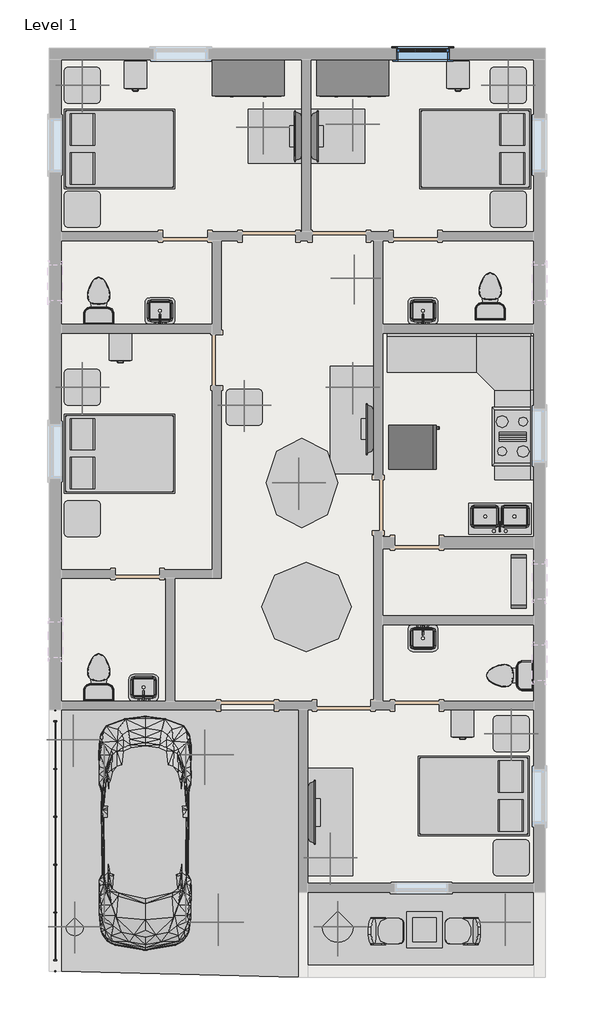
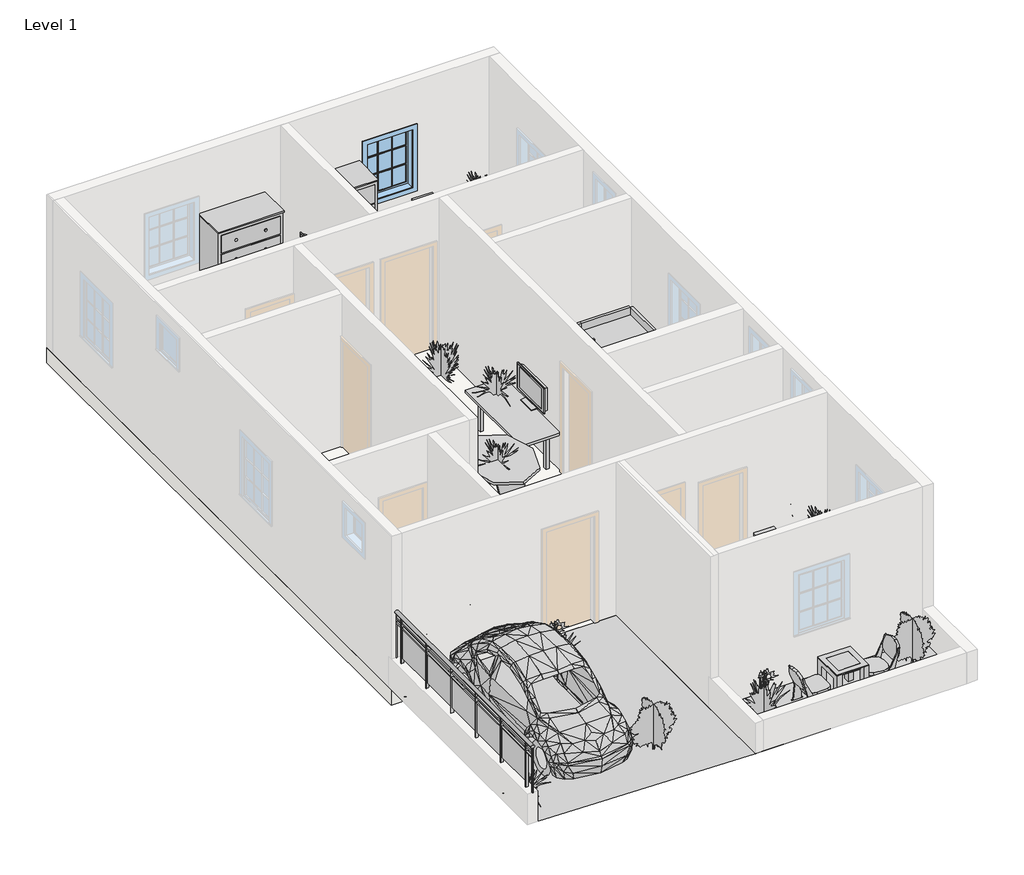
# One storey, part 2 of 2: 34 furniture elements, 17 geographic elements, 13 flow terminals, 5 proxies, 1 railing, 1 slab, 1 window.
"""IFC4 building model written with IfcOpenShell, lengths in millimetres."""

from ifc_helpers import new_model, si_unit, point, frame, origin, place, context, project, spatial, polyline, ellipse_curve, trimmed, outline, extrude, triangles, transform, mapped, element, save
from ifc_brep_helpers import plane_surface, extruded_surface, advanced_brep
from components import proxy_bb1e6e30, rpc_beetle_rpc_beetle_3ce7ba48, proxy_a13a33b2, flow_terminal_accce45a, flow_terminal_a53be723, flow_terminal_62a433f7, toilet_domestic_3d_toilet_domestic_3d_f7549cf7, toilet_domestic_3d_toilet_domestic_3d_183bbd19, furniture_c8abb964, furniture_bb55ed6b, furniture_9fa109b2, furniture_3d1d9cbc, furniture_417d203a, furniture_56245f3a, furniture_7a3aaa4f, furniture_b5c51a22, furniture_bbcc68ce, furniture_743965d2, furniture_31d08a24, furniture_4d44e21c, furniture_a5b052b6, furniture_125de5a1, rpc_plant_tropical_55f6ff97, rpc_plant_tropical_agave_1_5_93a2a214, rpc_plant_tropical_dagger_2_80c14bd7, rpc_plant_tropical_jungle_flame_3_9c4808c2, window_29c06734

model = new_model("IFC4")

# Units and contexts
model_context = context("Model", 3, world=origin())
ifc_project = project(units=[si_unit("LENGTHUNIT", "METRE", prefix="MILLI")], contexts=[model_context])

# Site, building, storey
site = spatial("IfcSite", under=ifc_project)
building = spatial("IfcBuilding", under=site)
storey = spatial("IfcBuildingStorey", under=building, Name="Level 1", Elevation=0.0)

# Proxies
placement = place(None, origin())
element("IfcBuildingElementProxy", 1, Name="Building Element Proxy", at=placement, inside=storey, context=model_context, shape_type="Tessellation", body=[
    triangles([(-16415.7270721, 2158.1188522, 0.0), (-12173.9266846, 2158.1188522, 0.0), (-12173.9266846, -2388.4812447, 0.0), (-16212.5266846, -2286.8811962, 0.0)], [[1, 4, 2], [3, 2, 4]], closed=False),
])
element("IfcBuildingElementProxy", 2, Name="Building Element Proxy", at=placement, inside=storey, context=model_context, shape_type="Tessellation", body=[
    triangles([(-12173.9266846, -940.6812447, 0.0), (-7982.9266846, -940.6812447, 0.0), (-7982.9266846, -2388.4812447, 0.0), (-12173.9266846, -2388.4812447, 0.0)], [[1, 4, 2], [3, 2, 4]], closed=False),
])
proxy_shape = proxy_bb1e6e30(model_context)
element("IfcBuildingElementProxy", 3, Name="Cook Top-4 Unit : 36\" x 20\"", ObjectType="Cook Top-4 Unit : 36\" x 20\"", at=placement, inside=storey, context=model_context, shape_type="MappedRepresentation", body=[
    mapped(proxy_shape, transform((-8541.7267032, 6806.3187882, 0.0), x_axis=(0.0, -1.0000000000000004, 0.0), y_axis=(1.0000000000000004, 0.0, 0.0), z_axis=(0.0, 0.0, 1.0))),
])
rpc_beetle_rpc_beetle_shape = rpc_beetle_rpc_beetle_3ce7ba48(model_context)
element("IfcBuildingElementProxy", 4, Name="RPC Beetle : RPC Beetle", ObjectType="RPC Beetle : RPC Beetle", at=placement, inside=storey, context=model_context, shape_type="MappedRepresentation", body=[
    mapped(rpc_beetle_rpc_beetle_shape, transform((-14790.1267032, 1294.5187882, 0.0), x_axis=(-1.0, 0.0, 0.0), y_axis=(0.0, -1.0, 0.0), z_axis=(0.0, 0.0, 1.0))),
])
proxy_2_shape = proxy_a13a33b2(model_context)
element("IfcBuildingElementProxy", 5, Name="Refrigerator : 30\" x 32\" RH", ObjectType="Refrigerator : 30\" x 32\" RH", at=placement, inside=storey, context=model_context, shape_type="MappedRepresentation", body=[
    mapped(proxy_2_shape, transform((-10260.9892032, 6620.9698167, 0.0), x_axis=(0.0, 1.0000000000000002, 0.0), y_axis=(-1.0000000000000002, 0.0, 0.0), z_axis=(0.0, 0.0, 1.0))),
])

# Flow terminals
flow_terminal_shape = flow_terminal_accce45a(model_context)
element("IfcFlowTerminal", 6, ObjectType="Floor Drain - Round : 5\" Strainer - 2\" Drain", at=placement, inside=storey, context=model_context, shape_type="MappedRepresentation", body=[
    mapped(flow_terminal_shape, transform((-15933.1267032, 9854.3187882, 0.0), x_axis=(1.0, 0.0, 0.0), y_axis=(0.0, 1.0, 0.0), z_axis=(0.0, 0.0, 1.0))),
])
element("IfcFlowTerminal", 7, ObjectType="Floor Drain - Round : 5\" Strainer - 2\" Drain", at=placement, inside=storey, context=model_context, shape_type="MappedRepresentation", body=[
    mapped(flow_terminal_shape, transform((-9329.1267032, 9828.9187882, 0.0), x_axis=(1.0, 0.0, 0.0), y_axis=(0.0, 1.0, 0.0), z_axis=(0.0, 0.0, 1.0))),
])
element("IfcFlowTerminal", 8, ObjectType="Floor Drain - Round : 5\" Strainer - 2\" Drain", at=placement, inside=storey, context=model_context, shape_type="MappedRepresentation", body=[
    mapped(flow_terminal_shape, transform((-15704.5267032, 3910.7187882, 0.0), x_axis=(1.0, 0.0, 0.0), y_axis=(0.0, 1.0, 0.0), z_axis=(0.0, 0.0, 1.0))),
])
element("IfcFlowTerminal", 9, ObjectType="Floor Drain - Round : 5\" Strainer - 2\" Drain", at=placement, inside=storey, context=model_context, shape_type="MappedRepresentation", body=[
    mapped(flow_terminal_shape, transform((-9252.9267032, 3351.9187882, 0.0), x_axis=(1.0, 0.0, 0.0), y_axis=(0.0, 1.0, 0.0), z_axis=(0.0, 0.0, 1.0))),
])
flow_terminal_2_shape = flow_terminal_a53be723(model_context)
element("IfcFlowTerminal", 10, ObjectType="Sink Kitchen-Double : 42\" x 21\"", at=placement, inside=storey, context=model_context, shape_type="MappedRepresentation", body=[
    mapped(flow_terminal_2_shape, transform((-8741.9374626, 5411.6641893, 0.0), x_axis=(-1.0000000000000004, 0.0, 0.0), y_axis=(0.0, -1.0000000000000004, 0.0), z_axis=(0.0, 0.0, 1.0))),
])
flow_terminal_3_shape = flow_terminal_62a433f7(model_context)
element("IfcFlowTerminal", 11, ObjectType="Sink Vanity-Square : 20\" x 18\"", at=placement, inside=storey, context=model_context, shape_type="MappedRepresentation", body=[
    mapped(flow_terminal_3_shape, transform((-14520.4374626, 8891.4641893, 0.0), x_axis=(-0.9999999999999999, 0.0, 0.0), y_axis=(0.0, -0.9999999999999999, 0.0), z_axis=(0.0, 0.0, 1.0))),
])
element("IfcFlowTerminal", 12, ObjectType="Sink Vanity-Square : 20\" x 18\"", at=placement, inside=storey, context=model_context, shape_type="MappedRepresentation", body=[
    mapped(flow_terminal_3_shape, transform((-10050.0374626, 8891.4641893, 0.0), x_axis=(-1.0, 0.0, 0.0), y_axis=(0.0, -1.0, 0.0), z_axis=(0.0, 0.0, 1.0))),
])
element("IfcFlowTerminal", 13, ObjectType="Sink Vanity-Square : 20\" x 18\"", at=placement, inside=storey, context=model_context, shape_type="MappedRepresentation", body=[
    mapped(flow_terminal_3_shape, transform((-14799.8374626, 2490.6641893, 0.0), x_axis=(-1.0000000000000002, 0.0, 0.0), y_axis=(0.0, -1.0000000000000002, 0.0), z_axis=(0.0, 0.0, 1.0))),
])
element("IfcFlowTerminal", 14, ObjectType="Sink Vanity-Square : 20\" x 18\"", at=placement, inside=storey, context=model_context, shape_type="MappedRepresentation", body=[
    mapped(flow_terminal_3_shape, transform((-10081.4159437, 3425.7733871, 0.0), x_axis=(1.0, 0.0, 0.0), y_axis=(0.0, 1.0, 0.0), z_axis=(0.0, 0.0, 1.0))),
])
toilet_domestic_3d_toilet_domestic_3d_shape = toilet_domestic_3d_toilet_domestic_3d_f7549cf7(model_context)
toilet_domestic_3d_toilet_domestic_3d_2_shape = toilet_domestic_3d_toilet_domestic_3d_183bbd19(model_context)
element("IfcFlowTerminal", 15, ObjectType="Toilet-Domestic-3D : Toilet-Domestic-3D", at=placement, inside=storey, context=model_context, shape_type="MappedRepresentation", body=[
    mapped(toilet_domestic_3d_toilet_domestic_3d_shape, transform((-15577.5267032, 9206.0148155, 0.0), x_axis=(-1.0000000000000002, 0.0, 0.0), y_axis=(0.0, -1.0000000000000002, 0.0), z_axis=(0.0, 0.0, 1.0))),
    mapped(toilet_domestic_3d_toilet_domestic_3d_2_shape, transform((-15577.5267032, 9206.0148155, 0.0), x_axis=(-1.0000000000000002, 0.0, 0.0), y_axis=(0.0, -1.0000000000000002, 0.0), z_axis=(0.0, 0.0, 1.0))),
])
element("IfcFlowTerminal", 16, ObjectType="Toilet-Domestic-3D : Toilet-Domestic-3D", at=placement, inside=storey, context=model_context, shape_type="MappedRepresentation", body=[
    mapped(toilet_domestic_3d_toilet_domestic_3d_shape, transform((-8922.7267032, 9282.2148155, 0.0), x_axis=(-0.9999999999999998, 0.0, 0.0), y_axis=(0.0, -0.9999999999999998, 0.0), z_axis=(0.0, 0.0, 1.0))),
    mapped(toilet_domestic_3d_toilet_domestic_3d_2_shape, transform((-8922.7267032, 9282.2148155, 0.0), x_axis=(-0.9999999999999998, 0.0, 0.0), y_axis=(0.0, -0.9999999999999998, 0.0), z_axis=(0.0, 0.0, 1.0))),
])
element("IfcFlowTerminal", 17, ObjectType="Toilet-Domestic-3D : Toilet-Domestic-3D", at=placement, inside=storey, context=model_context, shape_type="MappedRepresentation", body=[
    mapped(toilet_domestic_3d_toilet_domestic_3d_shape, transform((-15577.5267032, 2805.2148155, 0.0), x_axis=(-1.0000000000000002, 0.0, 0.0), y_axis=(0.0, -1.0000000000000002, 0.0), z_axis=(0.0, 0.0, 1.0))),
    mapped(toilet_domestic_3d_toilet_domestic_3d_2_shape, transform((-15577.5267032, 2805.2148155, 0.0), x_axis=(-1.0000000000000002, 0.0, 0.0), y_axis=(0.0, -1.0000000000000002, 0.0), z_axis=(0.0, 0.0, 1.0))),
])
element("IfcFlowTerminal", 18, ObjectType="Toilet-Domestic-3D : Toilet-Domestic-3D", at=placement, inside=storey, context=model_context, shape_type="MappedRepresentation", body=[
    mapped(toilet_domestic_3d_toilet_domestic_3d_shape, transform((-8680.8227305, 2742.3187882, 0.0), x_axis=(0.0, -1.0000000000000002, 0.0), y_axis=(1.0000000000000002, 0.0, 0.0), z_axis=(0.0, 0.0, 1.0))),
    mapped(toilet_domestic_3d_toilet_domestic_3d_2_shape, transform((-8680.8227305, 2742.3187882, 0.0), x_axis=(0.0, -1.0000000000000002, 0.0), y_axis=(1.0000000000000002, 0.0, 0.0), z_axis=(0.0, 0.0, 1.0))),
])

# Furniture
furniture_shape = furniture_c8abb964(model_context)
element("IfcFurniture", 19, ObjectType="Bed-Box : Double 53\" x 74\"", at=placement, inside=storey, context=model_context, shape_type="MappedRepresentation", body=[
    mapped(furniture_shape, transform((-15456.3562114, 11356.6663292, 0.0), x_axis=(0.0, 1.0, 0.0), y_axis=(-1.0, 0.0, 0.0), z_axis=(0.0, 0.0, 1.0))),
])
element("IfcFurniture", 20, ObjectType="Bed-Box : Double 53\" x 74\"", at=placement, inside=storey, context=model_context, shape_type="MappedRepresentation", body=[
    mapped(furniture_shape, transform((-8942.297195, 12034.9712472, 0.0), x_axis=(0.0, -1.0, 0.0), y_axis=(1.0, 0.0, 0.0), z_axis=(0.0, 0.0, 1.0))),
])
element("IfcFurniture", 21, ObjectType="Bed-Box : Double 53\" x 74\"", at=placement, inside=storey, context=model_context, shape_type="MappedRepresentation", body=[
    mapped(furniture_shape, transform((-15456.3562114, 6175.0663292, 0.0), x_axis=(0.0, 1.0, 0.0), y_axis=(-1.0, 0.0, 0.0), z_axis=(0.0, 0.0, 1.0))),
])
element("IfcFurniture", 22, ObjectType="Bed-Box : Double 53\" x 74\"", at=placement, inside=storey, context=model_context, shape_type="MappedRepresentation", body=[
    mapped(furniture_shape, transform((-8967.697195, 1036.7712472, 0.0), x_axis=(0.0, -1.0, 0.0), y_axis=(1.0, 0.0, 0.0), z_axis=(0.0, 0.0, 1.0))),
])
furniture_2_shape = furniture_bb55ed6b(model_context)
element("IfcFurniture", 23, ObjectType="Cabinet-File 2 Drawer : 15\" x 18\"", at=placement, inside=storey, context=model_context, shape_type="MappedRepresentation", body=[
    mapped(furniture_2_shape, transform((-14827.3302561, 13095.2530883, 0.0), x_axis=(1.0, 0.0, 0.0), y_axis=(0.0, 1.0, 0.0), z_axis=(0.0, 0.0, 1.0))),
])
element("IfcFurniture", 24, ObjectType="Cabinet-File 2 Drawer : 15\" x 18\"", at=placement, inside=storey, context=model_context, shape_type="MappedRepresentation", body=[
    mapped(furniture_2_shape, transform((-9340.9302561, 13095.2530883, 0.0), x_axis=(1.0, 0.0, 0.0), y_axis=(0.0, 1.0, 0.0), z_axis=(0.0, 0.0, 1.0))),
])
element("IfcFurniture", 25, ObjectType="Cabinet-File 2 Drawer : 15\" x 18\"", at=placement, inside=storey, context=model_context, shape_type="MappedRepresentation", body=[
    mapped(furniture_2_shape, transform((-9264.7302561, 2071.6530883, 0.0), x_axis=(1.0, 0.0, 0.0), y_axis=(0.0, 1.0, 0.0), z_axis=(0.0, 0.0, 1.0))),
])
element("IfcFurniture", 26, ObjectType="Cabinet-File 2 Drawer : 15\" x 18\"", at=placement, inside=storey, context=model_context, shape_type="MappedRepresentation", body=[
    mapped(furniture_2_shape, transform((-15081.3302561, 8472.4530883, 0.0), x_axis=(1.0, 0.0, 0.0), y_axis=(0.0, 1.0, 0.0), z_axis=(0.0, 0.0, 1.0))),
])
furniture_3_shape = furniture_9fa109b2(model_context)
element("IfcFurniture", 27, ObjectType="Dresser : 48\" x 72\" x 24\"", at=placement, inside=storey, context=model_context, shape_type="MappedRepresentation", body=[
    mapped(furniture_3_shape, transform((-12768.3334433, 13265.4817423, 0.0), x_axis=(1.0, 0.0, 0.0), y_axis=(0.0, 1.0, 0.0), z_axis=(0.0, 0.0, 1.0))),
])
element("IfcFurniture", 28, ObjectType="Dresser : 48\" x 72\" x 24\"", at=placement, inside=storey, context=model_context, shape_type="MappedRepresentation", body=[
    mapped(furniture_3_shape, transform((-10990.3334433, 13265.4817423, 0.0), x_axis=(1.0, 0.0, 0.0), y_axis=(0.0, 1.0, 0.0), z_axis=(0.0, 0.0, 1.0))),
])
furniture_4_shape = furniture_3d1d9cbc(model_context)
element("IfcFurniture", 29, ObjectType="Seating-Auditorium : 18\" x 24\" x 30\"", at=placement, inside=storey, context=model_context, shape_type="MappedRepresentation", body=[
    mapped(furniture_4_shape, transform((-9190.0512933, -1761.8090807, 0.0), x_axis=(0.0, 1.0000000000000002, 0.0), y_axis=(-1.0000000000000002, 0.0, 0.0), z_axis=(0.0, 0.0, 1.0))),
])
element("IfcFurniture", 30, ObjectType="Seating-Auditorium : 18\" x 24\" x 30\"", at=placement, inside=storey, context=model_context, shape_type="MappedRepresentation", body=[
    mapped(furniture_4_shape, transform((-10890.602113, -1440.353343, 0.0), x_axis=(0.0, -1.0000000000000004, 0.0), y_axis=(1.0000000000000004, 0.0, 0.0), z_axis=(0.0, 0.0, 1.0))),
])
furniture_5_shape = furniture_417d203a(model_context)
element("IfcFurniture", 31, ObjectType="Shelving : 36\" x 10\" x 72\"", at=placement, inside=storey, context=model_context, shape_type="MappedRepresentation", body=[
    mapped(furniture_5_shape, transform((-8744.9267032, 4342.5187882, 0.0), x_axis=(0.0, 1.0000000000000002, 0.0), y_axis=(-1.0000000000000002, 0.0, 0.0), z_axis=(0.0, 0.0, 1.0))),
])
furniture_6_shape = furniture_56245f3a(model_context)
element("IfcFurniture", 32, ObjectType="TV - Flat Screen : 32\"", at=placement, inside=storey, context=model_context, shape_type="MappedRepresentation", body=[
    mapped(furniture_6_shape, transform((-12181.6653268, 11907.774274, 914.4), x_axis=(0.0, -1.0000000000000004, 0.0), y_axis=(1.0000000000000004, 0.0, 0.0), z_axis=(0.0, 0.0, 1.0))),
])
element("IfcFurniture", 33, ObjectType="TV - Flat Screen : 32\"", at=placement, inside=storey, context=model_context, shape_type="MappedRepresentation", body=[
    mapped(furniture_6_shape, transform((-11912.1880795, 11915.6633023, 914.4), x_axis=(0.0, 1.0000000000000002, 0.0), y_axis=(-1.0000000000000002, 0.0, 0.0), z_axis=(0.0, 0.0, 1.0))),
])
element("IfcFurniture", 34, ObjectType="TV - Flat Screen : 32\"", at=placement, inside=storey, context=model_context, shape_type="MappedRepresentation", body=[
    mapped(furniture_6_shape, transform((-10962.4653268, 6929.374274, 914.4), x_axis=(0.0, -1.0000000000000004, 0.0), y_axis=(1.0000000000000004, 0.0, 0.0), z_axis=(0.0, 0.0, 1.0))),
])
furniture_7_shape = furniture_7a3aaa4f(model_context)
element("IfcFurniture", 35, ObjectType="TV - Flat Screen : 42\"", at=placement, inside=storey, context=model_context, shape_type="MappedRepresentation", body=[
    mapped(furniture_7_shape, transform((-11962.9880795, 422.1633023, 914.4), x_axis=(0.0, 1.0000000000000002, 0.0), y_axis=(-1.0000000000000002, 0.0, 0.0), z_axis=(0.0, 0.0, 1.0))),
])
furniture_8_shape = furniture_b5c51a22(model_context)
element("IfcFurniture", 36, ObjectType="Table-Coffee : 24\" x 24\" x 24\"", at=placement, inside=storey, context=model_context, shape_type="MappedRepresentation", body=[
    mapped(furniture_8_shape, transform((-10058.5924698, -1670.8922896, 0.0), x_axis=(1.0, 0.0, 0.0), y_axis=(0.0, 1.0, 0.0), z_axis=(0.0, 0.0, 1.0))),
])
furniture_9_shape = furniture_bbcc68ce(model_context)
element("IfcFurniture", 37, ObjectType="Table-Dining Round w Chairs : 60\" Diameter", at=placement, inside=storey, context=model_context, shape_type="MappedRepresentation", body=[
    mapped(furniture_9_shape, transform((-12150.6086704, 4095.5974767, 0.0), x_axis=(1.0, 0.0, 0.0), y_axis=(0.0, 1.0, 0.0), z_axis=(0.0, 0.0, 1.0))),
])
furniture_10_shape = furniture_743965d2(model_context)
element("IfcFurniture", 38, ObjectType="Table-Ellipse : 60\" x 48\"", at=placement, inside=storey, context=model_context, shape_type="MappedRepresentation", body=[
    mapped(furniture_10_shape, transform((-12123.1267032, 6018.9187882, 0.0), x_axis=(0.0, 1.0, 0.0), y_axis=(-1.0, 0.0, 0.0), z_axis=(0.0, 0.0, 1.0))),
])
furniture_11_shape = furniture_31d08a24(model_context)
element("IfcFurniture", 39, ObjectType="Table-End : 24\" x 24\"", at=placement, inside=storey, context=model_context, shape_type="MappedRepresentation", body=[
    mapped(furniture_11_shape, transform((-16165.4603335, 12622.9187882, 0.0), x_axis=(1.0, 0.0, 0.0), y_axis=(0.0, 1.0, 0.0), z_axis=(0.0, 0.0, 1.0))),
])
element("IfcFurniture", 40, ObjectType="Table-End : 24\" x 24\"", at=placement, inside=storey, context=model_context, shape_type="MappedRepresentation", body=[
    mapped(furniture_11_shape, transform((-16165.4603335, 10514.7187882, 0.0), x_axis=(1.0, 0.0, 0.0), y_axis=(0.0, 1.0, 0.0), z_axis=(0.0, 0.0, 1.0))),
])
element("IfcFurniture", 41, ObjectType="Table-End : 24\" x 24\"", at=placement, inside=storey, context=model_context, shape_type="MappedRepresentation", body=[
    mapped(furniture_11_shape, transform((-8926.4603335, 12622.9187882, 0.0), x_axis=(1.0, 0.0, 0.0), y_axis=(0.0, 1.0, 0.0), z_axis=(0.0, 0.0, 1.0))),
])
element("IfcFurniture", 42, ObjectType="Table-End : 24\" x 24\"", at=placement, inside=storey, context=model_context, shape_type="MappedRepresentation", body=[
    mapped(furniture_11_shape, transform((-8926.4603335, 10514.7187882, 0.0), x_axis=(1.0, 0.0, 0.0), y_axis=(0.0, 1.0, 0.0), z_axis=(0.0, 0.0, 1.0))),
])
element("IfcFurniture", 43, ObjectType="Table-End : 24\" x 24\"", at=placement, inside=storey, context=model_context, shape_type="MappedRepresentation", body=[
    mapped(furniture_11_shape, transform((-16165.4603335, 7492.1187882, 0.0), x_axis=(1.0, 0.0, 0.0), y_axis=(0.0, 1.0, 0.0), z_axis=(0.0, 0.0, 1.0))),
])
element("IfcFurniture", 44, ObjectType="Table-End : 24\" x 24\"", at=placement, inside=storey, context=model_context, shape_type="MappedRepresentation", body=[
    mapped(furniture_11_shape, transform((-16165.4603335, 5256.9187882, 0.0), x_axis=(1.0, 0.0, 0.0), y_axis=(0.0, 1.0, 0.0), z_axis=(0.0, 0.0, 1.0))),
])
element("IfcFurniture", 45, ObjectType="Table-End : 24\" x 24\"", at=placement, inside=storey, context=model_context, shape_type="MappedRepresentation", body=[
    mapped(furniture_11_shape, transform((-8875.6603335, 1599.3187882, 0.0), x_axis=(1.0, 0.0, 0.0), y_axis=(0.0, 1.0, 0.0), z_axis=(0.0, 0.0, 1.0))),
])
element("IfcFurniture", 46, ObjectType="Table-End : 24\" x 24\"", at=placement, inside=storey, context=model_context, shape_type="MappedRepresentation", body=[
    mapped(furniture_11_shape, transform((-8875.6603335, -508.8812118, 0.0), x_axis=(1.0, 0.0, 0.0), y_axis=(0.0, 1.0, 0.0), z_axis=(0.0, 0.0, 1.0))),
])
element("IfcFurniture", 47, ObjectType="Table-End : 24\" x 24\"", at=placement, inside=storey, context=model_context, shape_type="MappedRepresentation", body=[
    mapped(furniture_11_shape, transform((-13409.5603335, 7149.2187882, 0.0), x_axis=(1.0, 0.0, 0.0), y_axis=(0.0, 1.0, 0.0), z_axis=(0.0, 0.0, 1.0))),
])
furniture_12_shape = furniture_4d44e21c(model_context)
element("IfcFurniture", 48, ObjectType="Table-Rectangular : 36\" x 36\"", at=placement, inside=storey, context=model_context, shape_type="MappedRepresentation", body=[
    mapped(furniture_12_shape, transform((-11513.5267032, 11911.7187882, 0.0), x_axis=(1.0, 0.0, 0.0), y_axis=(0.0, 1.0, 0.0), z_axis=(0.0, 0.0, 1.0))),
])
element("IfcFurniture", 49, ObjectType="Table-Rectangular : 36\" x 36\"", at=placement, inside=storey, context=model_context, shape_type="MappedRepresentation", body=[
    mapped(furniture_12_shape, transform((-12580.3267032, 11911.7187882, 0.0), x_axis=(1.0, 0.0, 0.0), y_axis=(0.0, 1.0, 0.0), z_axis=(0.0, 0.0, 1.0))),
])
furniture_13_shape = furniture_a5b052b6(model_context)
element("IfcFurniture", 50, ObjectType="Table-Rectangular : 72\" x 30\"", at=placement, inside=storey, context=model_context, shape_type="MappedRepresentation", body=[
    mapped(furniture_13_shape, transform((-11640.5267032, 253.1187882, 0.0), x_axis=(0.0, 1.0, 0.0), y_axis=(-1.0, 0.0, 0.0), z_axis=(0.0, 0.0, 1.0))),
])
element("IfcFurniture", 51, ObjectType="Table-Rectangular : 72\" x 30\"", at=placement, inside=storey, context=model_context, shape_type="MappedRepresentation", body=[
    mapped(furniture_13_shape, transform((-11259.5267032, 7085.7187882, 0.0), x_axis=(0.0, 1.0, 0.0), y_axis=(-1.0, 0.0, 0.0), z_axis=(0.0, 0.0, 1.0))),
])
furniture_14_shape = furniture_125de5a1(model_context)
element("IfcFurniture", 52, ObjectType="Work Station Cubicle : 96\" x 96\"", at=placement, inside=storey, context=model_context, shape_type="MappedRepresentation", body=[
    mapped(furniture_14_shape, transform((-7691.1036955, 8427.187036, 0.0), x_axis=(0.0, -1.0000000000000004, 0.0), y_axis=(1.0000000000000004, 0.0, 0.0), z_axis=(0.0, 0.0, 1.0))),
])

# Geographic elements
rpc_plant_tropical_shape = rpc_plant_tropical_55f6ff97(model_context)
element("IfcGeographicElement", 53, ObjectType="RPC Plant - Tropical", at=placement, inside=storey, context=model_context, shape_type="MappedRepresentation", body=[
    mapped(rpc_plant_tropical_shape, transform((-11513.5267032, -1524.8812118, 0.0), x_axis=(1.0, 0.0, 0.0), y_axis=(0.0, 1.0, 0.0), z_axis=(0.0, 0.0, 1.0))),
])
element("IfcGeographicElement", 54, ObjectType="RPC Plant - Tropical", at=placement, inside=storey, context=model_context, shape_type="MappedRepresentation", body=[
    mapped(rpc_plant_tropical_shape, transform((-13774.1267032, 1396.1187882, 0.0), x_axis=(1.0, 0.0, 0.0), y_axis=(0.0, 1.0, 0.0), z_axis=(0.0, 0.0, 1.0))),
])
rpc_plant_tropical_agave_1_5_shape = rpc_plant_tropical_agave_1_5_93a2a214(model_context)
element("IfcGeographicElement", 55, ObjectType="RPC Plant - Tropical : Agave - 1.5'", at=placement, inside=storey, context=model_context, shape_type="MappedRepresentation", body=[
    mapped(rpc_plant_tropical_agave_1_5_shape, transform((-15856.9267032, 12775.3187882, 609.6), x_axis=(1.0, 0.0, 0.0), y_axis=(0.0, 1.0, 0.0), z_axis=(0.0, 0.0, 1.0))),
])
element("IfcGeographicElement", 56, ObjectType="RPC Plant - Tropical : Agave - 1.5'", at=placement, inside=storey, context=model_context, shape_type="MappedRepresentation", body=[
    mapped(rpc_plant_tropical_agave_1_5_shape, transform((-8617.9267032, 12775.3187882, 609.6), x_axis=(1.0, 0.0, 0.0), y_axis=(0.0, 1.0, 0.0), z_axis=(0.0, 0.0, 1.0))),
])
element("IfcGeographicElement", 57, ObjectType="RPC Plant - Tropical : Agave - 1.5'", at=placement, inside=storey, context=model_context, shape_type="MappedRepresentation", body=[
    mapped(rpc_plant_tropical_agave_1_5_shape, transform((-15856.9267032, 7644.5187882, 609.6), x_axis=(1.0, 0.0, 0.0), y_axis=(0.0, 1.0, 0.0), z_axis=(0.0, 0.0, 1.0))),
])
element("IfcGeographicElement", 58, ObjectType="RPC Plant - Tropical : Agave - 1.5'", at=placement, inside=storey, context=model_context, shape_type="MappedRepresentation", body=[
    mapped(rpc_plant_tropical_agave_1_5_shape, transform((-8567.1267032, 1751.7187882, 609.6), x_axis=(1.0, 0.0, 0.0), y_axis=(0.0, 1.0, 0.0), z_axis=(0.0, 0.0, 1.0))),
])
element("IfcGeographicElement", 59, ObjectType="RPC Plant - Tropical : Agave - 1.5'", at=placement, inside=storey, context=model_context, shape_type="MappedRepresentation", body=[
    mapped(rpc_plant_tropical_agave_1_5_shape, transform((-13101.0267032, 7339.7187882, 609.6), x_axis=(1.0, 0.0, 0.0), y_axis=(0.0, 1.0, 0.0), z_axis=(0.0, 0.0, 1.0))),
])
element("IfcGeographicElement", 60, ObjectType="RPC Plant - Tropical : Agave - 1.5'", at=placement, inside=storey, context=model_context, shape_type="MappedRepresentation", body=[
    mapped(rpc_plant_tropical_agave_1_5_shape, transform((-12173.9267032, 6018.9187882, 609.6), x_axis=(1.0, 0.0, 0.0), y_axis=(0.0, 1.0, 0.0), z_axis=(0.0, 0.0, 1.0))),
])
element("IfcGeographicElement", 61, ObjectType="RPC Plant - Tropical : Agave - 1.5'", at=placement, inside=storey, context=model_context, shape_type="MappedRepresentation", body=[
    mapped(rpc_plant_tropical_agave_1_5_shape, transform((-16009.3267032, 1650.1187882, 0.0), x_axis=(1.0, 0.0, 0.0), y_axis=(0.0, 1.0, 0.0), z_axis=(0.0, 0.0, 1.0))),
])
element("IfcGeographicElement", 62, ObjectType="RPC Plant - Tropical : Agave - 1.5'", at=placement, inside=storey, context=model_context, shape_type="MappedRepresentation", body=[
    mapped(rpc_plant_tropical_agave_1_5_shape, transform((-15983.9267032, -1524.8812118, 0.0), x_axis=(1.0, 0.0, 0.0), y_axis=(0.0, 1.0, 0.0), z_axis=(0.0, 0.0, 1.0))),
])
element("IfcGeographicElement", 63, ObjectType="RPC Plant - Tropical : Agave - 1.5'", at=placement, inside=storey, context=model_context, shape_type="MappedRepresentation", body=[
    mapped(rpc_plant_tropical_agave_1_5_shape, transform((-11640.5267032, -356.4812118, 762.0), x_axis=(1.0, 0.0, 0.0), y_axis=(0.0, 1.0, 0.0), z_axis=(0.0, 0.0, 1.0))),
])
element("IfcGeographicElement", 64, ObjectType="RPC Plant - Tropical : Agave - 1.5'", at=placement, inside=storey, context=model_context, shape_type="MappedRepresentation", body=[
    mapped(rpc_plant_tropical_agave_1_5_shape, transform((-11259.5267032, 7644.5187882, 762.0), x_axis=(1.0, 0.0, 0.0), y_axis=(0.0, 1.0, 0.0), z_axis=(0.0, 0.0, 1.0))),
])
element("IfcGeographicElement", 65, ObjectType="RPC Plant - Tropical : Agave - 1.5'", at=placement, inside=storey, context=model_context, shape_type="MappedRepresentation", body=[
    mapped(rpc_plant_tropical_agave_1_5_shape, transform((-11259.5267032, 12114.9187882, 762.0), x_axis=(1.0, 0.0, 0.0), y_axis=(0.0, 1.0, 0.0), z_axis=(0.0, 0.0, 1.0))),
])
element("IfcGeographicElement", 66, ObjectType="RPC Plant - Tropical : Agave - 1.5'", at=placement, inside=storey, context=model_context, shape_type="MappedRepresentation", body=[
    mapped(rpc_plant_tropical_agave_1_5_shape, transform((-12783.5267032, 12064.1187882, 762.0), x_axis=(1.0, 0.0, 0.0), y_axis=(0.0, 1.0, 0.0), z_axis=(0.0, 0.0, 1.0))),
])
rpc_plant_tropical_dagger_2_shape = rpc_plant_tropical_dagger_2_80c14bd7(model_context)
element("IfcGeographicElement", 67, ObjectType="RPC Plant - Tropical : Dagger - 2'", at=placement, inside=storey, context=model_context, shape_type="MappedRepresentation", body=[
    mapped(rpc_plant_tropical_dagger_2_shape, transform((-11234.1267032, 9498.7187882, 0.0), x_axis=(1.0, 0.0, 0.0), y_axis=(0.0, 1.0, 0.0), z_axis=(0.0, 0.0, 1.0))),
])
rpc_plant_tropical_jungle_flame_3_shape = rpc_plant_tropical_jungle_flame_3_9c4808c2(model_context)
element("IfcGeographicElement", 68, ObjectType="RPC Plant - Tropical : Jungle Flame - 3'", at=placement, inside=storey, context=model_context, shape_type="MappedRepresentation", body=[
    mapped(rpc_plant_tropical_jungle_flame_3_shape, transform((-8668.7267032, -1448.6812118, 0.0), x_axis=(1.0, 0.0, 0.0), y_axis=(0.0, 1.0, 0.0), z_axis=(0.0, 0.0, 1.0))),
])
element("IfcGeographicElement", 69, ObjectType="RPC Plant - Tropical : Jungle Flame - 3'", at=placement, inside=storey, context=model_context, shape_type="MappedRepresentation", body=[
    mapped(rpc_plant_tropical_jungle_flame_3_shape, transform((-13545.5267032, -1448.6812118, 0.0), x_axis=(1.0, 0.0, 0.0), y_axis=(0.0, 1.0, 0.0), z_axis=(0.0, 0.0, 1.0))),
])

# Railing
element("IfcRailing", 70, ObjectType="Glass Panel - Bottom Fill", at=placement, inside=storey, context=model_context, shape_type="SolidModel", body=[
    advanced_brep(
    [(-16276.0267032, 2158.1187882, 1524.0), (-16352.2267032, 2158.1187882, 1524.0), (-16276.0267032, -2286.8812118, 1524.0), (-16352.2267032, -2286.8812118, 1524.0)],
    [
        (0, 1, ellipse_curve(frame((-16314.1267032, 2158.1187882, 1524.0), z_axis=(0.0, 1.0, 0.0), x_axis=(-1.0, 0.0, 0.0)), 38.1, 28.575)),
        (1, 0, ellipse_curve(frame((-16314.1267032, 2158.1187882, 1524.0), z_axis=(0.0, 1.0, 0.0), x_axis=(-1.0, 0.0, 0.0)), 38.1, 28.575)),
        (2, 3, ellipse_curve(frame((-16314.1267032, -2286.8812118, 1524.0), z_axis=(0.0, -1.0, 0.0), x_axis=(-1.0, 0.0, 0.0)), 38.1, 28.575)),
        (3, 2, ellipse_curve(frame((-16314.1267032, -2286.8812118, 1524.0), z_axis=(0.0, -1.0, 0.0), x_axis=(-1.0, 0.0, 0.0)), 38.1, 28.575)),
        (0, 2),
        (3, 1),
    ],
    [
        plane_surface(frame((-16314.1267032, 2158.1187882, 1524.0), z_axis=(0.0, 1.0, 0.0), x_axis=(0.0, 0.0, -1.0))),
        plane_surface(frame((-16314.1267032, -2286.8812118, 1524.0), z_axis=(0.0, -1.0, 0.0), x_axis=(0.0, 0.0, -1.0))),
        extruded_surface(trimmed(ellipse_curve(frame((-16314.1267032, -2286.8812118, 1524.0), z_axis=(0.0, 1.0, 0.0), x_axis=(-1.0, 0.0, 0.0)), 38.1, 28.575), [point((-16276.0267032, -2286.8812118, 1524.0))], [point((-16352.2267032, -2286.8812118, 1524.0))], True, "CARTESIAN"), (0.0, 4445.0, 0.0), 4445.0),
        extruded_surface(trimmed(ellipse_curve(frame((-16314.1267032, -2286.8812118, 1524.0), z_axis=(0.0, 1.0, 0.0), x_axis=(-1.0, 0.0, 0.0)), 38.1, 28.575), [point((-16352.2267032, -2286.8812118, 1524.0))], [point((-16276.0267032, -2286.8812118, 1524.0))], True, "CARTESIAN"), (0.0, 4445.0, 0.0), 4445.0),
    ],
    [
        (0, [[1, 2]]),
        (1, [[3, 4]]),
        (2, [[-1, 5, -4, 6]]),
        (3, [[-2, -6, -3, -5]]),
    ],
),
    extrude(outline(polyline([(-16326.8267032, 2158.1187882), (-16301.4267032, 2158.1187882), (-16301.4267032, -2286.8812118), (-16326.8267032, -2286.8812118), (-16326.8267032, 2158.1187882)])), frame((0.0, 0.0, 1409.7), z_axis=(0.0, 0.0, 1.0), x_axis=(1.0, 0.0, 0.0)), (0.0, 0.0, 1.0), 25.4),
    extrude(outline(polyline([(-16326.8267032, 2158.1187882), (-16301.4267032, 2158.1187882), (-16301.4267032, -2286.8812118), (-16326.8267032, -2286.8812118), (-16326.8267032, 2158.1187882)])), frame((0.0, 0.0, 1308.1), z_axis=(0.0, 0.0, 1.0), x_axis=(1.0, 0.0, 0.0)), (0.0, 0.0, 1.0), 25.4),
    extrude(outline(polyline([(-16339.5267032, -2090.0312118), (-16288.7267032, -2090.0312118), (-16288.7267032, -2102.7312118), (-16339.5267032, -2102.7312118), (-16339.5267032, -2090.0312118)])), frame((0.0, 0.0, 609.6), z_axis=(0.0, 0.0, 1.0), x_axis=(1.0, 0.0, 0.0)), (0.0, 0.0, 1.0), 885.6788223),
    extrude(outline(polyline([(-16307.5915462, -1283.5812118), (-16307.5915462, -2096.3812118), (-16313.9415462, -2096.3812118), (-16313.9415462, -1283.5812118), (-16307.5915462, -1283.5812118)])), frame((0.0, 0.0, 711.2), z_axis=(0.0, 0.0, 1.0), x_axis=(1.0, 0.0, 0.0)), (0.0, 0.0, 1.0), 596.9),
    extrude(outline(polyline([(-16339.5267032, -1277.2312118), (-16288.7267032, -1277.2312118), (-16288.7267032, -1289.9312118), (-16339.5267032, -1289.9312118), (-16339.5267032, -1277.2312118)])), frame((0.0, 0.0, 609.6), z_axis=(0.0, 0.0, 1.0), x_axis=(1.0, 0.0, 0.0)), (0.0, 0.0, 1.0), 885.6788223),
    extrude(outline(polyline([(-16307.5915462, -470.7812118), (-16307.5915462, -1283.5812118), (-16313.9415462, -1283.5812118), (-16313.9415462, -470.7812118), (-16307.5915462, -470.7812118)])), frame((0.0, 0.0, 711.2), z_axis=(0.0, 0.0, 1.0), x_axis=(1.0, 0.0, 0.0)), (0.0, 0.0, 1.0), 596.9),
    extrude(outline(polyline([(-16339.5267032, -464.4312118), (-16288.7267032, -464.4312118), (-16288.7267032, -477.1312118), (-16339.5267032, -477.1312118), (-16339.5267032, -464.4312118)])), frame((0.0, 0.0, 609.6), z_axis=(0.0, 0.0, 1.0), x_axis=(1.0, 0.0, 0.0)), (0.0, 0.0, 1.0), 885.6788223),
    extrude(outline(polyline([(-16307.5915462, 342.0187882), (-16307.5915462, -470.7812118), (-16313.9415462, -470.7812118), (-16313.9415462, 342.0187882), (-16307.5915462, 342.0187882)])), frame((0.0, 0.0, 711.2), z_axis=(0.0, 0.0, 1.0), x_axis=(1.0, 0.0, 0.0)), (0.0, 0.0, 1.0), 596.9),
    extrude(outline(polyline([(-16339.5267032, 348.3687882), (-16288.7267032, 348.3687882), (-16288.7267032, 335.6687882), (-16339.5267032, 335.6687882), (-16339.5267032, 348.3687882)])), frame((0.0, 0.0, 609.6), z_axis=(0.0, 0.0, 1.0), x_axis=(1.0, 0.0, 0.0)), (0.0, 0.0, 1.0), 885.6788223),
    extrude(outline(polyline([(-16307.5915462, 1154.8187882), (-16307.5915462, 342.0187882), (-16313.9415462, 342.0187882), (-16313.9415462, 1154.8187882), (-16307.5915462, 1154.8187882)])), frame((0.0, 0.0, 711.2), z_axis=(0.0, 0.0, 1.0), x_axis=(1.0, 0.0, 0.0)), (0.0, 0.0, 1.0), 596.9),
    extrude(outline(polyline([(-16339.5267032, 1161.1687882), (-16288.7267032, 1161.1687882), (-16288.7267032, 1148.4687882), (-16339.5267032, 1148.4687882), (-16339.5267032, 1161.1687882)])), frame((0.0, 0.0, 609.6), z_axis=(0.0, 0.0, 1.0), x_axis=(1.0, 0.0, 0.0)), (0.0, 0.0, 1.0), 885.6788223),
    extrude(outline(polyline([(-16307.5915462, 1967.6187882), (-16307.5915462, 1154.8187882), (-16313.9415462, 1154.8187882), (-16313.9415462, 1967.6187882), (-16307.5915462, 1967.6187882)])), frame((0.0, 0.0, 711.2), z_axis=(0.0, 0.0, 1.0), x_axis=(1.0, 0.0, 0.0)), (0.0, 0.0, 1.0), 596.9),
    extrude(outline(polyline([(-16339.5267032, 1973.9687882), (-16288.7267032, 1973.9687882), (-16288.7267032, 1961.2687882), (-16339.5267032, 1961.2687882), (-16339.5267032, 1973.9687882)])), frame((0.0, 0.0, 609.6), z_axis=(0.0, 0.0, 1.0), x_axis=(1.0, 0.0, 0.0)), (0.0, 0.0, 1.0), 885.6788223),
    extrude(outline(polyline([(-16323.6517032, -2274.1812118), (-16304.6017032, -2274.1812118), (-16304.6017032, -2293.2312118), (-16323.6517032, -2293.2312118), (-16323.6517032, -2274.1812118)])), frame((0.0, 0.0, 609.6), z_axis=(0.0, 0.0, 1.0), x_axis=(1.0, 0.0, 0.0)), (0.0, 0.0, 1.0), 885.6788223),
    extrude(outline(polyline([(-16323.6517032, 2164.4687882), (-16304.6017032, 2164.4687882), (-16304.6017032, 2145.4187882), (-16323.6517032, 2145.4187882), (-16323.6517032, 2164.4687882)])), frame((0.0, 0.0, 609.6), z_axis=(0.0, 0.0, 1.0), x_axis=(1.0, 0.0, 0.0)), (0.0, 0.0, 1.0), 885.6788223),
])

# Slab
element("IfcSlab", 71, ObjectType="Generic - 12\"", at=placement, inside=storey, context=model_context, shape_type="SweptSolid", body=[
    extrude(outline(polyline([(-7982.9267032, 13410.3187882), (-7982.9267032, -940.6812118), (-12173.9267032, -940.6812118), (-12173.9267032, 2158.1187882), (-16415.7267032, 2158.1187882), (-16415.7267032, 13410.3187882), (-7982.9267032, 13410.3187882)])), frame((0.0, 0.0, -304.8), z_axis=(0.0, 0.0, 1.0), x_axis=(1.0, 0.0, 0.0)), (0.0, 0.0, 1.0), 304.8),
])

# Window
window_shape = window_29c06734(model_context)
element("IfcWindow", 72, ObjectType="Casement 3x3 with Trim : 36\" x 48\"", at=placement, inside=storey, context=model_context, shape_type="MappedRepresentation", body=[
    mapped(window_shape, transform((-10065.7267032, 13308.7187882, 0.0), x_axis=(1.0, 0.0, 0.0), y_axis=(0.0, 1.0, 0.0), z_axis=(0.0, 0.0, 1.0))),
])

save(model, "model.ifc")

# Revit data of these elements
# Type "Cook Top-4 Unit : 36\" x 20\""
#   Assembly Code = "E1090400"
#   Depth = 2' - 0"
#   Width = 3' - 0"
#   Burner Material = Steel, Chrome Plated
#   Cooktop Material = Steel, Polished
#   Default Elevation = 0
# Type "RPC Beetle : RPC Beetle"
#   built-in parameter 1005195 = "RPC-16-0U6E-L4EG-ENH1-J3KF-SVEL-0TX4-C0"
#   Height = 0
# Type "Refrigerator : 30\" x 32\" RH"
#   Label = "REF."
#   Assembly Code = "E1090400"
#   Depth = 2' - 7 3/4"
#   Handle = 2' - 3"
#   Height = 5' - 10"
#   Rear Clearance = 0' - 2"
#   Top Door Height = 1' - 8"
#   Width = 2' - 5 3/8"
#   Material = Steel, Paint Finish, Ivory, Glossy
#   Default Elevation = 0
# Type "Floor Drain - Round : 5\" Strainer - 2\" Drain"
#   WFU = 2
#   Strainer Height = 0' - 3 1/4"
#   Strainer Radius = 0' - 2 1/2"
#   Strainer Diameter = 0' - 5"
#   Radius 6 = 0' - 0 5/8"
#   Radius 5 = 0' - 1 1/4"
#   Radius 4 = 0' - 1 7/8"
#   Radius 2 = 0' - 3.04167"
#   Radius 1 = 0' - 2.02083"
#   Radius 3 = 0' - 2 1/32"
#   Pipe Radius = 1"
#   Pipe Diameter = 2"
#   Height 2 = 0' - 0.725"
#   Height 1 = 0' - 1 13/16"
#   Body Radius = 0' - 4 1/16"
#   Body Height = 0' - 3 5/8"
#   Body Diameter = 0' - 8 1/8"
#   Drain Material = none
#   HWFU = 0
#   Default Elevation = 0
#   CWFU = 0
# Type "Sink Kitchen-Double : 42\" x 21\""
#   Assembly Code = "D2010410"
#   Counter Height = 3' - 0"
#   Depth = 1' - 9"
#   Width = 3' - 6"
#   Faucet Material = Steel, Polished
#   Sink Material = Steel, Polished
#   Default Elevation = 0
# Type "Sink Vanity-Square : 20\" x 18\""
#   Assembly Code = "D2010400"
#   Counter Height = 2' - 7"
#   Depth = 1' - 6"
#   Width = 1' - 8"
#   Basin Material = Porcelain, Linen
#   Faucet Material = Steel, Polished
#   Default Elevation = 0
# Type "Toilet-Domestic-3D : Toilet-Domestic-3D"
#   Assembly Code = "D2010110"
#   Toilet - Bowl/Basin Material = Porcelain, Linen
#   Toilet - Seat Material = Laminate, Linen, Matte
#   Default Elevation = 0
# Type "Bed-Box : Double 53\" x 74\""
#   Assembly Code = "E2020200"
#   Length = 6' - 2"
#   Width = 4' - 5"
#   Frame Material = Birch
#   Mattress Material = Linen, White
#   Default Elevation = 0
# Type "Cabinet-File 2 Drawer : 15\" x 18\""
#   Assembly Code = "E2020200"
#   Depth = 1' - 6"
#   Height = 2' - 5"
#   Width = 1' - 3"
#   Cabinet Material = Steel, Paint Finish, Ivory, Glossy
#   Handle Material = Steel, Chrome Plated
#   Default Elevation = 0
# Type "Dresser : 48\" x 72\" x 24\""
#   Assembly Code = "E2020200"
#   Depth = 2' - 0"
#   Height = 6' - 0"
#   Width = 4' - 0"
#   Dresser Material = Laminate - Ivory, Glossy
#   Drawer Material = Laminate, Ivory, Matte
#   Knob Material = Cherry
#   Default Elevation = 0
# Type "Seating-Auditorium : 18\" x 24\" x 30\""
#   Assembly Code = "E2020200"
#   Seat Material = Linen, Beige
#   Frame Material = Steel, Paint Finish, Dark Gray, Matte
#   Default Elevation = 0
# Type "Shelving : 36\" x 10\" x 72\""
#   Assembly Code = "E2020200"
#   Depth = 0' - 10"
#   Height = 6' - 0"
#   Width = 3' - 0"
#   Shelving Unit Material = Birch
#   Default Elevation = 0
# Type "TV - Flat Screen : 32\""
#   SinAng = 0' - 0.0193"
#   L = 2' - 3.79372"
#   H = 1' - 3.6354"
#   Thickness = 0' - 4.33071"
#   Diagonal = 2' - 7.88976"
#   CosAng = 0' - 0.03431"
#   Stand [instance default] = yes
#   Default Elevation = 0
# Type "TV - Flat Screen : 42\""
#   SinAng = 0' - 0.0193"
#   L = 3' - 0.71517"
#   H = 1' - 8.65418"
#   Thickness = 0' - 4.33071"
#   Diagonal = 3' - 6.12598"
#   CosAng = 0' - 0.03431"
#   Stand [instance default] = yes
#   Default Elevation = 0
# Type "Table-Coffee : 24\" x 24\" x 24\""
#   Assembly Code = "E2020200"
#   Height = 2' - 0"
#   Length = 2' - 0"
#   Width = 2' - 0"
#   Top Material = none
#   Frame Material = none
#   Default Elevation = 0
# Type "Table-Dining Round w Chairs : 60\" Diameter"
#   Assembly Code = "E2020200"
#   Radius = 2' - 6"
#   Diameter = 5' - 0"
#   Height = 2' - 6"
#   Chairs = 6
#   Base Material = Pine
#   Top Material = Laminate, Linen, Matte
#   Default Elevation = 0
# Type "Table-Ellipse : 60\" x 48\""
#   Assembly Code = "E2020200"
#   Half Width = 2' - 0"
#   Half Length = 2' - 6"
#   Height = 2' - 6"
#   Length = 5' - 0"
#   Width = 4' - 0"
#   Base Material = Birch
#   Top Material = Birch
#   Default Elevation = 0
# Type "Table-End : 24\" x 24\""
#   Assembly Code = "E2020200"
#   Height = 2' - 0"
#   Length = 2' - 0"
#   Width = 2' - 0"
#   Base Material = Birch
#   Top Material = Laminate, Ivory, Matte
#   Default Elevation = 0
# Type "Table-Rectangular : 36\" x 36\""
#   Assembly Code = "E2020200"
#   Height = 2' - 6"
#   Length = 3' - 0"
#   Width = 3' - 0"
#   Base Material = Birch
#   Top Material = Birch
#   Default Elevation = 0
# Type "Table-Rectangular : 72\" x 30\""
#   Assembly Code = "E2020200"
#   Height = 2' - 6"
#   Length = 6' - 0"
#   Width = 2' - 6"
#   Base Material = Birch
#   Top Material = Birch
#   Default Elevation = 0
# Type "Work Station Cubicle : 96\" x 96\""
#   Assembly Code = "E2020"
#   Desktop Height = 2' - 6"
#   Desktop1 Width = 2' - 0"
#   Desktop2 Width = 2' - 0"
#   Panel Height = 3' - 0"
#   Panel1 Length = 5' - 0"
#   Panel2 Length = 5' - 0"
#   Cube Panel Material = Textile - Light Gray
#   Work Top Material = Laminate, Ivory, Matte
#   Default Elevation = 0
# Type "RPC Plant - Tropical"
#   built-in parameter 1005198 = "{2, 15},{39, RPC-16-FWM5-GM7X-C67P-4000-ST1L-LVER-AU},{1, 0},{1, 0},{2, 13},{1, 8},{5, Color},{1, 0},{1, 0},{3, 0.8},{3, 0.8},{3, 0.8},{1, 8},{7, BBoxMin},{1, 0},{1, 0},{1, 0},{1, 0},{1, 0},{1, 8},{7, BBoxMax},{1, 0},{1, 0},{1, 0},{1, 0},{1, 0},{2, 11},{9, RPCTypeId},{1, 0},{1, 0},{39, RPC-16-FWM5-GM7X-C67P-4000-ST1L-LVER-AU},{1, 6},{14, RPCPlantHeight},{1, 0},{1, 0},{1, 3},{2, 11},{7, keyword},{1, 0},{1, 0},{35, :RPCs:Shrubs [General]:Geometry:RPC},{2, 11},{8, category},{1, 0},{1, 0},{16, Shrubs [General]},{2, 11},{12, LocalizedUID},{1, 0},{1, 0},{10, Crane Lily},{2, 14},{6, Height},{1, 0},{1, 0},{1, 3},{1, 2},{16, Cast Reflections},{1, 0},{1, 0},{1, 0},{1, 2},{12, Cast Shadows},{1, 0},{1, 0},{1, 1},{1, 2},{9, Lock View},{1, 0},{1, 0},{1, 0},{1, 4},{5, ViewC},{1, 0},{1, 0},{1, 0},{21, assetlibrary_base.fbx},{1, 5},"
#   built-in parameter 1005195 = "RPC-16-FWM5-GM7X-C67P-4000-ST1L-LVER-AU"
#   Assembly Code = "G2050500"
#   Height = 3' - 0"
#   Default Elevation = 0
# Type "RPC Plant - Tropical : Agave - 1.5'"
#   built-in parameter 1005198 = "{2, 15},{39, RPC-16-G1GJ-63FX-7K5P-N000-ST1L-LVER-AU},{1, 0},{1, 0},{2, 13},{1, 8},{5, Color},{1, 0},{1, 0},{3, 0.8},{3, 0.8},{3, 0.8},{1, 8},{7, BBoxMin},{1, 0},{1, 0},{1, 0},{1, 0},{1, 0},{1, 8},{7, BBoxMax},{1, 0},{1, 0},{1, 0},{1, 0},{1, 0},{2, 11},{9, RPCTypeId},{1, 0},{1, 0},{39, RPC-16-G1GJ-63FX-7K5P-N000-ST1L-LVER-AU},{1, 6},{14, RPCPlantHeight},{1, 0},{1, 0},{3, 1.5},{2, 11},{7, keyword},{1, 0},{1, 0},{35, :RPCs:Plants [General]:Geometry:RPC},{2, 11},{8, category},{1, 0},{1, 0},{16, Plants [General]},{2, 11},{12, LocalizedUID},{1, 0},{1, 0},{5, Agave},{2, 14},{6, Height},{1, 0},{1, 0},{3, 1.5},{1, 2},{16, Cast Reflections},{1, 0},{1, 0},{1, 0},{1, 2},{12, Cast Shadows},{1, 0},{1, 0},{1, 1},{1, 2},{9, Lock View},{1, 0},{1, 0},{1, 0},{1, 4},{5, ViewC},{1, 0},{1, 0},{1, 0},{21, assetlibrary_base.fbx},{1, 5},"
#   built-in parameter 1005195 = "RPC-16-G1GJ-63FX-7K5P-N000-ST1L-LVER-AU"
#   Type Comments = "Agave"
#   Assembly Code = "G2050500"
#   Height = 1' - 6"
#   Default Elevation = 0
# Type "RPC Plant - Tropical : Dagger - 2'"
#   built-in parameter 1005198 = "{2, 15},{39, RPC-16-G3A7-NEG0-UH6H-J000-ST1L-LVER-AU},{1, 0},{1, 0},{2, 13},{1, 8},{5, Color},{1, 0},{1, 0},{3, 0.8},{3, 0.8},{3, 0.8},{1, 8},{7, BBoxMin},{1, 0},{1, 0},{1, 0},{1, 0},{1, 0},{1, 8},{7, BBoxMax},{1, 0},{1, 0},{1, 0},{1, 0},{1, 0},{2, 11},{9, RPCTypeId},{1, 0},{1, 0},{39, RPC-16-G3A7-NEG0-UH6H-J000-ST1L-LVER-AU},{1, 6},{14, RPCPlantHeight},{1, 0},{1, 0},{1, 2},{2, 11},{7, keyword},{1, 0},{1, 0},{35, :RPCs:Plants [General]:Geometry:RPC},{2, 11},{8, category},{1, 0},{1, 0},{16, Plants [General]},{2, 11},{12, LocalizedUID},{1, 0},{1, 0},{6, Dagger},{2, 14},{6, Height},{1, 0},{1, 0},{1, 2},{1, 2},{16, Cast Reflections},{1, 0},{1, 0},{1, 0},{1, 2},{12, Cast Shadows},{1, 0},{1, 0},{1, 1},{1, 2},{9, Lock View},{1, 0},{1, 0},{1, 0},{1, 4},{5, ViewC},{1, 0},{1, 0},{1, 0},{21, assetlibrary_base.fbx},{1, 5},"
#   built-in parameter 1005195 = "RPC-16-G3A7-NEG0-UH6H-J000-ST1L-LVER-AU"
#   Type Comments = "Dagger"
#   Assembly Code = "G2050500"
#   Height = 2' - 0"
#   Default Elevation = 0
# Type "RPC Plant - Tropical : Jungle Flame - 3'"
#   built-in parameter 1005198 = "{2, 15},{39, RPC-16-FUVJ-JWG0-MWGK-8000-ST1L-LVER-AU},{1, 0},{1, 0},{2, 13},{1, 8},{5, Color},{1, 0},{1, 0},{3, 0.8},{3, 0.8},{3, 0.8},{1, 8},{7, BBoxMin},{1, 0},{1, 0},{1, 0},{1, 0},{1, 0},{1, 8},{7, BBoxMax},{1, 0},{1, 0},{1, 0},{1, 0},{1, 0},{2, 11},{9, RPCTypeId},{1, 0},{1, 0},{39, RPC-16-FUVJ-JWG0-MWGK-8000-ST1L-LVER-AU},{1, 6},{14, RPCPlantHeight},{1, 0},{1, 0},{1, 3},{2, 11},{7, keyword},{1, 0},{1, 0},{35, :RPCs:Shrubs [General]:Geometry:RPC},{2, 11},{8, category},{1, 0},{1, 0},{16, Shrubs [General]},{2, 11},{12, LocalizedUID},{1, 0},{1, 0},{12, Jungle Flame},{2, 14},{6, Height},{1, 0},{1, 0},{1, 3},{1, 2},{16, Cast Reflections},{1, 0},{1, 0},{1, 0},{1, 2},{12, Cast Shadows},{1, 0},{1, 0},{1, 1},{1, 2},{9, Lock View},{1, 0},{1, 0},{1, 0},{1, 4},{5, ViewC},{1, 0},{1, 0},{1, 0},{21, assetlibrary_base.fbx},{1, 5},"
#   built-in parameter 1005195 = "RPC-16-FUVJ-JWG0-MWGK-8000-ST1L-LVER-AU"
#   Type Comments = "Jungle Flame"
#   Assembly Code = "G2050500"
#   Height = 3' - 0"
#   Default Elevation = 0
# Type "Glass Panel - Bottom Fill"
#   Assembly Code = "C2010400"
#   built-in parameter 1008612 = 0.0416667 (stored number, unit not read)
#   built-in parameter 1008611 = 0.0416667 (stored number, unit not read)
#   built-in parameter 1008609 = 0.333333 (stored number, unit not read)
#   built-in parameter 1008604 = 0.166667 (stored number, unit not read)
#   built-in parameter 1008603 = 0.166667 (stored number, unit not read)
#   Railing Height = 3' - 0"
#   built-in parameter 1008630 = 2
#   built-in parameter 1008610 = 2
#   built-in parameter 1008618 = Baluster - Square : 3/4"
# Type "Generic - 12\""
#   Assembly Code = "B1010"
#   Function = 0
#   Layers, outside or top first: 1' - 0" no material (function 1)
# Type "Casement 3x3 with Trim : 36\" x 48\""
#   Type Mark = "10"
#   Construction Type Id = "GSP4R"
#   Assembly Code = "B2020100"
#   Analytic Construction = "1/8 in Pilkington single glazing"
#   Visual Light Transmittance = 0.9
#   Solar Heat Gain Coefficient = 0.78
#   Heat Transfer Coefficient (U) = 0.6496 BTU/(h·ft²·°F)
#   Height = 4' - 0"
#   Default Sill Height = 3' - 0"
#   Trim Projection - Ext. = 0' - 0 1/2"
#   Trim Projection - Int. = 0' - 0 3/4"
#   Trim Width - Exterior = 0' - 3 1/2"
#   Trim Width - Interior = 0' - 3 1/2"
#   Width = 3' - 0"
#   Window Inset = 0' - 0 3/4"
#   Define Thermal Properties by = 1
#   Glass Pane Material = Glass
#   Sash Material = Sash
#   Trim Exterior Material = Trim
#   Trim Interior Material = Trim
#   Wall Closure = (empty or 0)
# Elements 1, 2 (IfcBuildingElementProxy)
#   Material = none
#   Phase Created = New Construction
# Element 3 (IfcBuildingElementProxy, "Cook Top-4 Unit : 36\" x 20\"")
#   Phase Created = New Construction
#   Materials on its faces: "Steel, Chrome Plated", "Steel, Polished"
# Element 4 (IfcBuildingElementProxy, "RPC Beetle : RPC Beetle")
#   Phase Created = New Construction
# Element 5 (IfcBuildingElementProxy, "Refrigerator : 30\" x 32\" RH")
#   Phase Created = New Construction
#   Materials on its faces: "Steel, Paint Finish, Ivory, Glossy", "Steel, Chrome Plated"
# Element 6 (IfcFlowTerminal, "Floor Drain - Round : 5\" Strainer - 2\" Drain")
#   Mark = "3"
#   Phase Created = New Construction
# Element 7 (IfcFlowTerminal, "Floor Drain - Round : 5\" Strainer - 2\" Drain")
#   Mark = "6"
#   Phase Created = New Construction
# Element 8 (IfcFlowTerminal, "Floor Drain - Round : 5\" Strainer - 2\" Drain")
#   Mark = "9"
#   Phase Created = New Construction
# Element 9 (IfcFlowTerminal, "Floor Drain - Round : 5\" Strainer - 2\" Drain")
#   Mark = "12"
#   Phase Created = New Construction
# Element 10 (IfcFlowTerminal, "Sink Kitchen-Double : 42\" x 21\"")
#   Mark = "13"
#   Phase Created = New Construction
#   Materials on its faces: "Steel, Polished"
# Element 11 (IfcFlowTerminal, "Sink Vanity-Square : 20\" x 18\"")
#   Mark = "2"
#   Phase Created = New Construction
#   Materials on its faces: "Porcelain, Linen", "Steel, Polished"
# Element 12 (IfcFlowTerminal, "Sink Vanity-Square : 20\" x 18\"")
#   Mark = "4"
#   Phase Created = New Construction
#   Materials on its faces: "Porcelain, Linen", "Steel, Polished"
# Element 13 (IfcFlowTerminal, "Sink Vanity-Square : 20\" x 18\"")
#   Mark = "7"
#   Phase Created = New Construction
#   Materials on its faces: "Porcelain, Linen", "Steel, Polished"
# Element 14 (IfcFlowTerminal, "Sink Vanity-Square : 20\" x 18\"")
#   Mark = "11"
#   Phase Created = New Construction
#   Materials on its faces: "Porcelain, Linen", "Steel, Polished"
# Element 15 (IfcFlowTerminal, "Toilet-Domestic-3D : Toilet-Domestic-3D")
#   Mark = "1"
#   Phase Created = New Construction
#   Materials on its faces: "Porcelain, Linen", "Laminate, Linen, Matte"
# Element 16 (IfcFlowTerminal, "Toilet-Domestic-3D : Toilet-Domestic-3D")
#   Mark = "5"
#   Phase Created = New Construction
#   Materials on its faces: "Porcelain, Linen", "Laminate, Linen, Matte"
# Element 17 (IfcFlowTerminal, "Toilet-Domestic-3D : Toilet-Domestic-3D")
#   Mark = "8"
#   Phase Created = New Construction
#   Materials on its faces: "Porcelain, Linen", "Laminate, Linen, Matte"
# Element 18 (IfcFlowTerminal, "Toilet-Domestic-3D : Toilet-Domestic-3D")
#   Mark = "10"
#   Phase Created = New Construction
#   Materials on its faces: "Porcelain, Linen", "Laminate, Linen, Matte"
# Elements 19, 20, 21, 22 (IfcFurniture, "Bed-Box : Double 53\" x 74\"")
#   Phase Created = New Construction
#   Materials on its faces: "Birch", "Linen, White"
# Elements 23, 24, 25, 26 (IfcFurniture, "Cabinet-File 2 Drawer : 15\" x 18\"")
#   Phase Created = New Construction
#   Materials on its faces: "Steel, Chrome Plated", "Steel, Paint Finish, Ivory, Glossy"
# Elements 27, 28 (IfcFurniture, "Dresser : 48\" x 72\" x 24\"")
#   Phase Created = New Construction
#   Materials on its faces: "Laminate, Ivory, Matte", "Cherry", "Laminate - Ivory, Glossy"
# Elements 29, 30 (IfcFurniture, "Seating-Auditorium : 18\" x 24\" x 30\"")
#   Phase Created = New Construction
#   Materials on its faces: "Steel, Paint Finish, Dark Gray, Matte", "Linen, Beige"
# Element 31 (IfcFurniture, "Shelving : 36\" x 10\" x 72\"")
#   Phase Created = New Construction
#   Materials on its faces: "Birch"
# Elements 32, 33, 34 (IfcFurniture, "TV - Flat Screen : 32\"")
#   Stand = yes
#   Phase Created = New Construction
#   Materials on its faces: "TV - Black", "TV - Glass", "TV - Screen"
# Element 35 (IfcFurniture, "TV - Flat Screen : 42\"")
#   Stand = yes
#   Phase Created = New Construction
#   Materials on its faces: "TV - Black", "TV - Glass", "TV - Screen"
# Element 36 (IfcFurniture, "Table-Coffee : 24\" x 24\" x 24\"")
#   Phase Created = New Construction
#   Materials on its faces: "Glass - Clear, Grey"
# Element 37 (IfcFurniture, "Table-Dining Round w Chairs : 60\" Diameter")
#   Phase Created = New Construction
#   Materials on its faces: "Pine", "Laminate, Linen, Matte"
# Element 38 (IfcFurniture, "Table-Ellipse : 60\" x 48\"")
#   Phase Created = New Construction
#   Materials on its faces: "Birch"
# Elements 39, 40, 41, 42, 43, 44, 45, 46, 47 (IfcFurniture, "Table-End : 24\" x 24\"")
#   Phase Created = New Construction
#   Materials on its faces: "Laminate, Ivory, Matte", "Birch"
# Elements 48, 49 (IfcFurniture, "Table-Rectangular : 36\" x 36\"")
#   Phase Created = New Construction
#   Materials on its faces: "Birch"
# Elements 50, 51 (IfcFurniture, "Table-Rectangular : 72\" x 30\"")
#   Phase Created = New Construction
#   Materials on its faces: "Birch"
# Element 52 (IfcFurniture, "Work Station Cubicle : 96\" x 96\"")
#   Phase Created = New Construction
#   Materials on its faces: "Textile - Light Gray", "Laminate, Ivory, Matte"
# Elements 53, 54 (IfcGeographicElement, "RPC Plant - Tropical")
#   Phase Created = New Construction
# Elements 55, 56, 57, 58, 59, 60, 61, 62, 63, 64, 65, 66 (IfcGeographicElement, "RPC Plant - Tropical : Agave - 1.5'")
#   Phase Created = New Construction
# Element 67 (IfcGeographicElement, "RPC Plant - Tropical : Dagger - 2'")
#   Phase Created = New Construction
# Elements 68, 69 (IfcGeographicElement, "RPC Plant - Tropical : Jungle Flame - 3'")
#   Phase Created = New Construction
# Element 70 (IfcRailing, "Glass Panel - Bottom Fill")
#   built-in parameter 1008621 = 2 (stored number, unit not read)
#   Phase Created = New Construction
#   Materials on its faces: "Glass"
# Element 71 (IfcSlab, "Generic - 12\"")
#   Height Offset From Level = 0' - 0"
#   Phase Created = New Construction
#   Materials on its faces: "Default Floor"
# Element 72 (IfcWindow, "Casement 3x3 with Trim : 36\" x 48\"")
#   Mark = "5"
#   Phase Created = New Construction
#   Materials on its faces: "Sash", "Glass", "Trim"
# Materials
#   "Steel, Chrome Plated": class "Metal", colour RGB 17 17 17, transparency 0, Description = "Chromiuim plated steel", Cost = 0
#   "Steel, Polished": class "Metal", colour RGB 57 57 57, transparency 0, Description = "Polished steel", Cost = 0
#   "Steel, Paint Finish, Ivory, Glossy": class "Metal", colour RGB 247 247 239, transparency 0, Description = "Steel, paint finish, ivory, glossy", Cost = 0
#   "Porcelain, Linen": class "Ceramic", colour RGB 249 239 230, transparency 0, Description = "Porcelain, linen", Cost = 0
